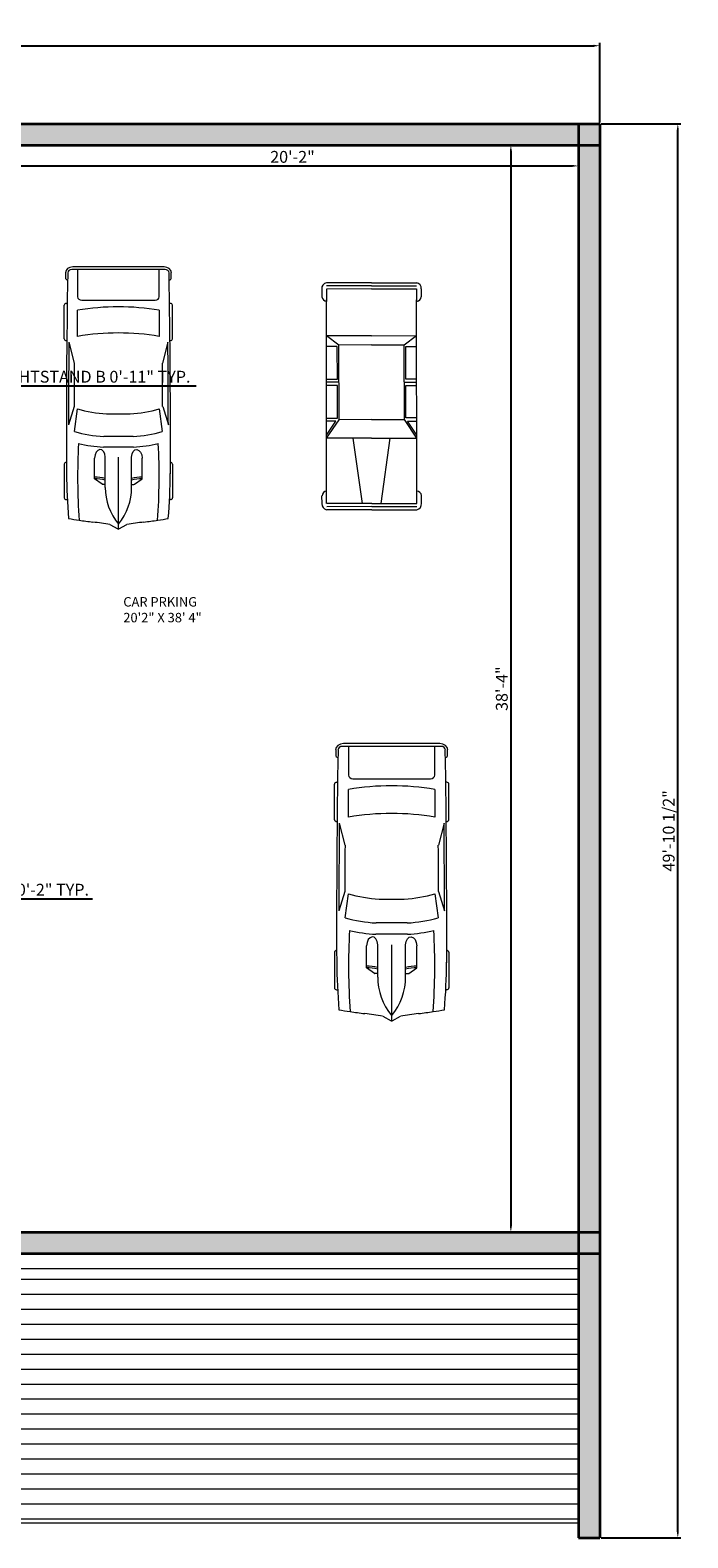
# Model space of a CAD drawing. Units: millimetres. Extents: x 2768 to 4359, y 795 to 1583.
# Tile 5 of 13: x 3226 to 3505, y 891 to 1529. Entities that reach past the tile are written whole.
import ezdxf

# ---------------------------------------------------------------- set-up
doc = ezdxf.new("R2010")
doc.units = ezdxf.units.MM
for name, color, linetype, lineweight in [('A-ANNO-DIMS', 90, 'Continuous', 18), ('A-AREA-IDEN', 190, 'Continuous', 18), ('A-DOOR-PATT', 251, 'Continuous', 13), ('A-WALL-PATT', 140, 'Continuous', 9), ('C-PKNG-VEHI', 50, 'Continuous', 13), ('iron shutter', 251, 'Continuous', 18), ('walls', 140, 'Continuous', 35)]:
    doc.layers.add(name, color=color, linetype=linetype, lineweight=lineweight)
doc.styles.get("Standard").update_dxf_attribs({"font": 'arial.ttf'})
doc.dimstyles.new('ISO-25', dxfattribs={"dimtxt": 5, "dimasz": 2.5, "dimexe": 1.25, "dimexo": 0.625, "dimtad": 1, "dimdec": 0, "dimlunit": 3, "dimtxsty": 'Standard', "dimcen": 2.5, "dimadec": 0, "dimazin": 0, "dimtfac": 1, "dimtdec": 0, "dimtmove": 0, "dimatfit": 3, "dimfxl": 1, "dimarcsym": 0})

# ---------------------------------------------------------------- blocks, each defined once
blk = doc.blocks.new('*U34')
for p, q in [((21.1, 37.4), (21.1, 36.8)), ((46.6, 38.9), (22.4, 38.9)), ((47.8, 37.4), (47.8, 37.4)), ((70, 31.5), (86.4, 29.4)), ((88, 31.9), (74.8, 35.9)), ((134.3, 35.6), (119.3, 31.8)), ((135.5, 37.1), (135.5, 37.4)), ((136.7, 38.9), (160.9, 38.9)), ((162.1, 37.4), (162.1, 36.8)), ((186.5, -33.5), (186.5, 33.5)), ((188.4, -32.8), (188.4, 32.8)), ((138.4, 29.4), (157.2, 29.4)), ((164.5, 26.4), (164.5, -26.4)), ((186.5, 29.4), (167, 29.4)), ((32.1, 9.5), (32.1, 11.2)), ((32.3, 11.6), (36.1, 17.2)), ((36.1, 17.2), (50.9, 17.2)), ((58.9, -10.8), (58.9, 10.8)), ((66.6, -10.5), (66.6, 10.5)), ((186.5, -10.5), (186.5, 10.5)), ((3.3, 6.1), (0.1, 0.4)), ((29.8, 9.5), (51.7, 9.5)), ((82.7, 8.5), (82.7, -8.5)), ((0, 0), (51.7, 0)), ((0.1, -0.4), (3.3, -6.1)), ((29.8, -9.5), (51.7, -9.5)), ((32.1, -9.5), (32.1, -11.2)), ((32.3, -11.6), (36.1, -17.2)), ((36.1, -17.2), (50.9, -17.2)), ((86.4, -29.4), (70, -31.5)), ((157.2, -29.4), (138.4, -29.4)), ((167, -29.4), (186.5, -29.4)), ((21.1, -37.4), (21.1, -36.8)), ((46.6, -38.9), (22.4, -38.9)), ((47.8, -37.4), (47.8, -37.4)), ((88, -31.9), (74.8, -35.9)), ((134.3, -35.6), (119.3, -31.8)), ((135.5, -37.1), (135.5, -37.4)), ((136.7, -38.9), (160.9, -38.9)), ((162.1, -37.4), (162.1, -36.8))]:
    blk.add_line(p, q)
for centre, major_axis, ratio, start_param, end_param in [((266, -27.5), (0, 313.3), 0.842304, 1.367076, 1.39176), ((41.2, -490.9), (0, 528.2), 0.842304, 0.00281, 0.075598), ((22.4, 37.4), (0, -1.48), 0.842304, 3.141593, 4.712389), ((64.5, -10555.6), (0, 10593), 0.842304, -0.013397, 0.002797), ((46.6, 37.4), (0, 1.48), 0.842304, -1.570796, 0), ((135.3, 5.4), (0, 81.8), 0.842304, 1.245306, 1.50788), ((64.5, -10555.6), (0, -10591.5), 0.842304, 3.133765, 3.140441), ((95.8, -3666.4), (0, -3698.2), 0.842304, 3.134049, 3.144098), ((136.7, 37.4), (0, -1.48), 0.842304, 3.141593, 4.712389), ((160.9, 37.4), (0, 1.48), 0.842304, -1.570796, 0), ((180.6, 35.8), (0, 2.22), 0.842304, -0.013017, 1.249894), ((64.5, -10556.4), (0, 10595.3), 0.842304, -0.013397, -0.013017), ((184, 32.8), (0, -5.25), 0.842304, 1.570796, 3.128196), ((184, 33.5), (0, -2.96), 0.842304, 1.570796, 3.128196), ((259.2, -27.5), (0, -305.3), 0.842304, 4.528606, 4.561838), ((37.5, -594), (0, -623.3), 0.842304, 3.096046, 3.200911), ((134.4, 5.4), (0, -89.8), 0.842304, 4.449482, 4.652344), ((149.6, 2.8), (0, -79.6), 0.842304, 4.372215, 4.640744), ((17.1, 0), (0, 147), 0.842304, 4.511394, 4.913384), ((35.9, 0), (0, 147), 0.842304, 4.511394, 4.913384), ((167, 26.4), (0, 2.96), 0.842304, 0, 1.570796), ((-204.5, 52.4), (0, -251), 0.842304, 1.385369, 1.434372), ((32.7, 11.2), (0, 0.74), 0.842304, 0.879714, 1.570796), ((13, 17), (0, 27.4), 0.842304, 4.435146, 4.718221), ((14.2, 17), (0, 27.4), 0.842304, 4.435146, 4.718221), ((50.8, 13.3), (6.34, -0.36), 0.603834, -1.395552, 1.581315), ((0.6, 0), (0, -0.74), 0.842304, 4.131459, 5.293319), ((29.8, -46.7), (0, 56.2), 0.842304, 0, 0.590319), ((-204.5, -52.4), (0, 251), 0.842304, -1.434372, -1.385369), ((29.8, 46.7), (0, 56.2), 0.842304, 2.551274, 3.141593), ((13, -17), (0, -27.4), 0.842304, 1.564964, 1.848039), ((14.2, -17), (0, -27.4), 0.842304, 1.564964, 1.848039), ((149.6, -2.8), (0, -79.6), 0.842304, -1.499151, -1.230623), ((259.2, 27.5), (0, 305.3), 0.842304, 1.721348, 1.754579), ((32.7, -11.2), (0, -0.74), 0.842304, 4.712389, 5.403472), ((134.4, -5.4), (0, -89.8), 0.842304, -1.510751, -1.307889), ((135.3, -5.4), (0, -81.8), 0.842304, -1.50788, -1.245306), ((266, 27.5), (0, 313.3), 0.842304, 1.749832, 1.774517), ((37.5, 594), (0, -623.3), 0.842304, -0.059319, 0.045547), ((167, -26.4), (0, -2.96), 0.842304, 4.712389, 6.283185), ((41.2, 490.9), (0, -528.2), 0.842304, -0.075598, -0.00281), ((22.4, -37.4), (0, 1.48), 0.842304, 1.570796, 3.141593), ((64.5, 10555.6), (0, 10593), 0.842304, 3.138796, 3.15499), ((46.6, -37.4), (0, -1.48), 0.842304, 0, 1.570796), ((64.5, 10555.6), (0, -10591.5), 0.842304, 0.001152, 0.007828), ((95.8, 3666.4), (0, -3698.2), 0.842304, -0.002505, 0.007544), ((136.7, -37.4), (0, -1.48), 0.842304, -1.570796, 0), ((160.9, -37.4), (0, 1.48), 0.842304, 3.141593, 4.712389), ((180.6, -35.8), (0, -2.22), 0.842304, -1.249894, 0.013017), ((64.5, 10556.4), (0, 10595.3), 0.842304, 3.15461, 3.15499), ((184, -32.8), (0, -5.25), 0.842304, 0.013397, 1.570796), ((184, -33.5), (0, 2.96), 0.842304, 3.15499, 4.712389)]:
    blk.add_ellipse(centre, major_axis=major_axis, ratio=ratio, start_param=start_param, end_param=end_param)
at = {"extrusion": (0, 0, -1)}
blk.add_ellipse((50.8, -13.3), major_axis=(6.34, 0.36), ratio=0.603834, start_param=-1.395552, end_param=1.581315, dxfattribs=at)
blk = doc.blocks.new('*U35')
for p, q in [((5.4, 42.3), (12.1, 42.3)), ((189.7, 42.3), (183, 42.3)), ((0.1, -0.4), (0.1, 38.3)), ((2.8, -0.4), (2.8, 38.3)), ((5.4, 38.3), (16.1, 38.3)), ((5.4, -0.4), (5.4, 38.2)), ((16.1, 38.3), (180.3, 38.3)), ((61.5, -0.4), (61.5, 38.3)), ((61.5, 38.3), (77.5, 27.6)), ((64.2, 38.3), (76.2, 30.3)), ((76.2, 30.3), (76.2, 38.3)), ((77.5, 27.6), (141.6, 27.6)), ((77.5, -0.4), (77.5, 27.6)), ((78.9, 38.3), (78.9, 29)), ((78.9, 29), (106.9, 29)), ((106.9, 29), (106.9, 38.3)), ((109.6, 27.6), (109.6, 38.3)), ((112.3, 38.3), (112.3, 29)), ((112.3, 29), (140.3, 29)), ((140.3, 29), (140.3, 38.3)), ((141.6, 27.6), (149.6, 38.3)), ((141.6, -0.4), (141.6, 27.6)), ((149.6, -0.4), (149.6, 38.3)), ((189.7, 38.3), (179, 38.3)), ((189.7, -0.4), (189.7, 38.2)), ((192.4, -0.4), (192.4, 38.3)), ((195, -0.4), (195, 38.3)), ((5.4, 7.6), (61.5, 15.6)), ((0.1, -0.4), (0.1, -39.2)), ((2.8, -0.4), (2.8, -39.1)), ((5.4, -0.4), (5.4, -39.1)), ((5.4, -8.4), (61.5, -16.4)), ((61.5, -0.4), (61.5, -39.1)), ((77.5, -0.4), (77.5, -28.5)), ((141.6, -0.4), (141.6, -28.5)), ((149.6, -0.4), (149.6, -39.1)), ((189.7, -0.4), (189.7, -39.1)), ((192.4, -0.4), (192.4, -39.1)), ((195, -0.4), (195, -39.2)), ((61.5, -39.1), (77.5, -28.5)), ((64.2, -39.1), (76.2, -31.1)), ((76.2, -31.1), (76.2, -39.1)), ((77.5, -28.5), (141.6, -28.5)), ((78.9, -39.1), (78.9, -29.8)), ((78.9, -29.8), (106.9, -29.8)), ((106.9, -29.8), (106.9, -39.1)), ((109.6, -28.5), (109.6, -39.1)), ((112.3, -29.8), (140.3, -29.8)), ((112.3, -39.1), (112.3, -29.8)), ((140.3, -29.8), (140.3, -39.1)), ((141.6, -28.5), (149.6, -39.1)), ((5.4, -39.1), (16.1, -39.1)), ((5.4, -43.1), (12.1, -43.1)), ((16.1, -39.1), (180.3, -39.1)), ((189.7, -39.1), (179, -39.1)), ((189.7, -43.1), (183, -43.1))]:
    blk.add_line(p, q)
for centre, radius, start, end in [((5.1, 37.3), 5.06, 85.6455, 168.0943), ((11.5, 37.6), 4.72, 8.1301, 81.87), ((183.7, 37.6), 4.72, 98.13, 171.8699), ((190.1, 37.3), 5.06, 11.9057, 94.3545), ((5.1, -38.1), 5.06, 191.9057, 274.3545), ((11.5, -38.5), 4.72, 278.13, 351.8699), ((183.7, -38.5), 4.72, 188.1301, 261.87), ((190.1, -38.1), 5.06, 265.6455, 348.0943)]:
    blk.add_arc(centre, radius, start, end)
blk = doc.blocks.new('*D36')
at = {"layer": 'A-ANNO-DIMS', "color": 0, "lineweight": -2, "transparency": 16777216}
for p, q in [((3216.41, 1480.21), (3216.41, 1470.35)), ((3458.41, 1480.21), (3458.41, 1470.35)), ((3218.91, 1471.6), (3455.91, 1471.6))]:
    blk.add_line(p, q, dxfattribs=at)
at = {"layer": 'A-ANNO-DIMS', "color": 0, "transparency": 16777216}
for points in [[(3218.91, 1472.02), (3218.91, 1471.19), (3216.41, 1471.6)], [(3455.91, 1472.02), (3455.91, 1471.19), (3458.41, 1471.6)]]:
    blk.add_solid(points, dxfattribs=at)
at = {"layer": 'Defpoints', "color": 0, "transparency": 16777216}
for p in [(3216.41, 1480.83), (3458.41, 1480.83), (3458.41, 1471.6)]:
    blk.add_point(p, dxfattribs=at)
at = {"layer": 'A-ANNO-DIMS', "color": 0, "transparency": 16777216, "insert": (3337.41, 1474.78), "char_height": 5, "attachment_point": 5}
blk.add_mtext('20\'-2"', dxfattribs=at)
blk = doc.blocks.new('*D37')
at = {"layer": 'A-ANNO-DIMS', "color": 0, "lineweight": -2, "transparency": 16777216}
for p, q in [((3428.05, 1480.41), (3431.06, 1480.41)), ((3429.81, 1477.91), (3429.81, 1022.91)), ((3428.05, 1020.41), (3431.06, 1020.41))]:
    blk.add_line(p, q, dxfattribs=at)
at = {"layer": 'A-ANNO-DIMS', "color": 0, "transparency": 16777216}
for points in [[(3429.39, 1477.91), (3430.23, 1477.91), (3429.81, 1480.41)], [(3429.39, 1022.91), (3430.23, 1022.91), (3429.81, 1020.41)]]:
    blk.add_solid(points, dxfattribs=at)
at = {"layer": 'Defpoints', "color": 0, "transparency": 16777216}
for p in [(3427.42, 1480.41), (3427.42, 1020.41), (3429.81, 1020.41)]:
    blk.add_point(p, dxfattribs=at)
at = {"layer": 'A-ANNO-DIMS', "color": 0, "transparency": 16777216, "insert": (3426.63, 1250.41), "char_height": 5, "attachment_point": 5, "rotation": 90}
blk.add_mtext('38\'-4"', dxfattribs=at)
blk = doc.blocks.new('*D119')
at = {"layer": 'A-ANNO-DIMS', "color": 0, "lineweight": -2, "transparency": 16777216}
for p, q in [((3193.99, 1379.55), (3193.99, 1377.29)), ((3196.49, 1378.54), (3202.37, 1378.54)), ((3204.87, 1379.55), (3204.87, 1377.29)), ((3204.87, 1378.54), (3296.68, 1378.54))]:
    blk.add_line(p, q, dxfattribs=at)
at = {"layer": 'A-ANNO-DIMS', "color": 0, "transparency": 16777216}
for points in [[(3196.49, 1378.96), (3196.49, 1378.13), (3193.99, 1378.54)], [(3202.37, 1378.96), (3202.37, 1378.13), (3204.87, 1378.54)]]:
    blk.add_solid(points, dxfattribs=at)
at = {"layer": 'Defpoints', "color": 0, "transparency": 16777216}
for p in [(3193.99, 1380.18), (3204.87, 1380.18), (3204.87, 1378.54)]:
    blk.add_point(p, dxfattribs=at)
at = {"layer": 'A-ANNO-DIMS', "color": 0, "transparency": 16777216, "insert": (3252.03, 1381.75), "char_height": 5, "attachment_point": 5}
blk.add_mtext('NIGHTSTAND B 0\'-11" TYP.', dxfattribs=at)
blk = doc.blocks.new('*D121')
at = {"layer": 'A-ANNO-DIMS', "color": 0, "lineweight": -2, "transparency": 16777216}
for p, q in [((3192.58, 1161.48), (3190.08, 1161.48)), ((3195.08, 1161.48), (3196.87, 1161.48)), ((3195.08, 1161.12), (3195.08, 1160.23)), ((3196.87, 1161.12), (3196.87, 1160.23)), ((3199.37, 1161.48), (3252.74, 1161.48))]:
    blk.add_line(p, q, dxfattribs=at)
at = {"layer": 'A-ANNO-DIMS', "color": 0, "transparency": 16777216}
for points in [[(3192.58, 1161.9), (3192.58, 1161.06), (3195.08, 1161.48)], [(3199.37, 1161.9), (3199.37, 1161.06), (3196.87, 1161.48)]]:
    blk.add_solid(points, dxfattribs=at)
at = {"layer": 'Defpoints', "color": 0, "transparency": 16777216}
for p in [(3195.08, 1161.75), (3196.87, 1161.75), (3196.87, 1161.48)]:
    blk.add_point(p, dxfattribs=at)
at = {"layer": 'A-ANNO-DIMS', "color": 0, "transparency": 16777216, "insert": (3227.3, 1164.69), "char_height": 5, "attachment_point": 5}
blk.add_mtext('RING 0\'-2" TYP.', dxfattribs=at)
blk = doc.blocks.new('*D125')
at = {"layer": 'A-ANNO-DIMS', "color": 0, "lineweight": -2, "transparency": 16777216}
for p, q in [((2811.41, 1490.03), (2811.41, 1523.71)), ((2813.91, 1522.46), (3464.91, 1522.46)), ((3467.41, 1490.03), (3467.41, 1523.71))]:
    blk.add_line(p, q, dxfattribs=at)
at = {"layer": 'A-ANNO-DIMS', "color": 0, "transparency": 16777216}
for points in [[(2813.91, 1522.87), (2813.91, 1522.04), (2811.41, 1522.46)], [(3464.91, 1522.87), (3464.91, 1522.04), (3467.41, 1522.46)]]:
    blk.add_solid(points, dxfattribs=at)
at = {"layer": 'Defpoints', "color": 0, "transparency": 16777216}
for p in [(3467.41, 1522.46), (2811.41, 1489.41), (3467.41, 1489.41)]:
    blk.add_point(p, dxfattribs=at)
at = {"layer": 'A-ANNO-DIMS', "color": 0, "transparency": 16777216, "insert": (3139.41, 1525.63), "char_height": 5, "attachment_point": 5}
blk.add_mtext('54\'-8"', dxfattribs=at)
blk = doc.blocks.new('*D126')
at = {"layer": 'A-ANNO-DIMS', "color": 0, "lineweight": -2, "transparency": 16777216}
for p, q in [((3468.03, 1489.41), (3501.71, 1489.41)), ((3500.46, 893.59), (3500.46, 1486.91)), ((3468.03, 891.09), (3501.71, 891.09))]:
    blk.add_line(p, q, dxfattribs=at)
at = {"layer": 'A-ANNO-DIMS', "color": 0, "transparency": 16777216}
for points in [[(3500.04, 1486.91), (3500.87, 1486.91), (3500.46, 1489.41)], [(3500.04, 893.59), (3500.87, 893.59), (3500.46, 891.09)]]:
    blk.add_solid(points, dxfattribs=at)
at = {"layer": 'Defpoints', "color": 0, "transparency": 16777216}
for p in [(3467.41, 1489.41), (3500.46, 1489.41), (3467.41, 891.09)]:
    blk.add_point(p, dxfattribs=at)
at = {"layer": 'A-ANNO-DIMS', "color": 0, "transparency": 16777216, "insert": (3497.25, 1190.25), "char_height": 5, "attachment_point": 5, "rotation": 90}
blk.add_mtext('49\'-10 1/2"', dxfattribs=at)

msp = doc.modelspace()

# ---------------------------------------------------------------- hatches: boundary and pattern name
at = {"layer": 'A-DOOR-PATT'}
h = msp.add_hatch(dxfattribs=at)
h.set_pattern_fill('ANSI31', color=256, scale=1.99444, angle=-45, style=0)
h.paths.add_polyline_path([(3216.41, 1005.07), (3458.41, 1005.07), (3458.41, 897.42), (3216.41, 897.42)])
at = {"layer": 'A-WALL-PATT'}
h = msp.add_hatch(color=256, dxfattribs=at)
h.dxf.hatch_style = 1
h.paths.add_polyline_path([(2820.41, 1480.41), (2811.41, 1480.41), (2811.41, 1360.41), (2820.41, 1360.41)])
h.paths.add_polyline_path([(2820.41, 1489.41), (2811.41, 1489.41), (2811.41, 1480.41), (2820.41, 1480.41)])
h.paths.add_polyline_path([(2845.83, 1489.41), (2820.41, 1489.41), (2820.41, 1480.41), (2845.83, 1480.41)])
h.paths.add_polyline_path([(2940.41, 1489.41), (2894.95, 1489.41), (2894.95, 1480.41), (2940.41, 1480.41)])
h.paths.add_polyline_path([(2949.41, 1489.41), (2940.41, 1489.41), (2940.41, 1480.41), (2949.41, 1480.41)])
h.paths.add_polyline_path([(2949.41, 1480.41), (2940.41, 1480.41), (2940.41, 1433.68), (2943.15, 1433.68), (2949.41, 1433.68)])
h.paths.add_polyline_path([(2964.2, 1489.41), (2949.41, 1489.41), (2949.41, 1480.41), (2964.2, 1480.41)])
h.paths.add_polyline_path([(3018.41, 1489.41), (3009.41, 1489.41), (3009.41, 1480.41), (3018.41, 1480.41)])
h.paths.add_polyline_path([(3009.41, 1489.41), (2990.92, 1489.41), (2990.92, 1480.41), (3009.41, 1480.41)])
h.paths.add_polyline_path([(3018.41, 1480.41), (3009.41, 1480.41), (3009.41, 1384.41), (3018.41, 1384.41)])
h.paths.add_polyline_path([(3009.41, 1384.41), (2949.41, 1384.41), (2949.41, 1375.41), (3009.41, 1375.41)])
h.paths.add_polyline_path([(3018.41, 1384.41), (3009.41, 1384.41), (3009.41, 1375.41), (3018.41, 1375.41)])
h.paths.add_polyline_path([(2949.41, 1384.41), (2940.41, 1384.41), (2940.41, 1375.41), (2949.41, 1375.41)])
h.paths.add_polyline_path([(2949.41, 1413.64, -0.075856), (2943.15, 1412.69), (2940.41, 1412.69), (2940.41, 1384.41), (2949.41, 1384.41)])
h.paths.add_polyline_path([(2949.41, 1375.41), (2940.41, 1375.41), (2940.41, 1360.41), (2949.41, 1360.41)])
h.paths.add_polyline_path([(2949.41, 1360.41), (2940.41, 1360.41), (2940.41, 1351.41), (2949.41, 1351.41)])
h.paths.add_polyline_path([(2940.41, 1360.41), (2929.82, 1360.41, -0.054277), (2930.46, 1354.53), (2930.46, 1351.41), (2940.41, 1351.41)])
h.paths.add_polyline_path([(2903.16, 1354.53), (2903.16, 1360.41), (2895.41, 1360.41), (2895.41, 1351.41), (2903.16, 1351.41)])
h.paths.add_polyline_path([(2886.41, 1360.41), (2820.41, 1360.41), (2820.41, 1351.41), (2886.41, 1351.41)])
h.paths.add_polyline_path([(2895.41, 1360.41), (2886.41, 1360.41), (2886.41, 1351.41), (2895.41, 1351.41)])
h.paths.add_polyline_path([(2820.41, 1360.41), (2811.41, 1360.41), (2811.41, 1351.41), (2820.41, 1351.41)])
h.paths.add_polyline_path([(2820.41, 1351.41), (2811.41, 1351.41), (2811.41, 1213.41), (2820.41, 1213.41)])
h.paths.add_polyline_path([(2886.41, 1213.41), (2820.41, 1213.41), (2820.41, 1204.41), (2886.41, 1204.41)])
h.paths.add_polyline_path([(2820.41, 1213.41), (2811.41, 1213.41), (2811.41, 1204.41), (2820.41, 1204.41)])
h.paths.add_polyline_path([(2895.41, 1302), (2886.41, 1302), (2886.41, 1264.47), (2895.41, 1264.47)])
h.paths.add_polyline_path([(2934.05, 1209.82), (2934.05, 1213.41), (2895.41, 1213.41), (2895.41, 1204.41), (2934.59, 1204.41, -0.049949)])
h.paths.add_polyline_path([(2895.41, 1213.41), (2886.41, 1213.41), (2886.41, 1204.41), (2895.41, 1204.41)])
h.paths.add_polyline_path([(3078.41, 1384.41), (3018.41, 1384.41), (3018.41, 1375.41), (3078.41, 1375.41)])
h.paths.add_polyline_path([(3087.41, 1433.68), (3084.62, 1433.68), (3078.41, 1433.68), (3078.41, 1384.41), (3087.41, 1384.41)])
h.paths.add_polyline_path([(3087.41, 1384.41), (3078.41, 1384.41), (3078.41, 1375.41), (3087.41, 1375.41)])
h.paths.add_polyline_path([(3087.41, 1375.41), (3078.41, 1375.41), (3078.41, 1360.41), (3087.41, 1360.41)])
h.paths.add_polyline_path([(3087.41, 1360.41), (3078.41, 1360.41), (3078.41, 1351.41), (3087.41, 1351.41)])
h.paths.add_polyline_path([(3093.5, 1360.41), (3087.41, 1360.41), (3087.41, 1351.41), (3093.5, 1351.41), (3093.5, 1353.18)])
h.paths.add_polyline_path([(3207.41, 1360.41), (3119.82, 1360.41, -0.067042), (3120.8, 1353.18), (3120.8, 1351.41), (3207.41, 1351.41)])
h.paths.add_polyline_path([(3216.41, 1480.41), (3207.41, 1480.41), (3207.41, 1360.41), (3216.41, 1360.41)])
h.paths.add_polyline_path([(3216.41, 1360.41), (3207.41, 1360.41), (3207.41, 1351.41), (3216.41, 1351.41)])
h.paths.add_polyline_path([(3216.41, 1489.41), (3207.41, 1489.41), (3207.41, 1480.41), (3216.41, 1480.41)])
h.paths.add_polyline_path([(3207.41, 1489.41), (3167.11, 1489.41), (3167.11, 1480.41), (3207.41, 1480.41)])
h.paths.add_polyline_path([(3118.27, 1489.41), (3087.41, 1489.41), (3087.41, 1480.41), (3118.27, 1480.41)])
h.paths.add_polyline_path([(3087.41, 1489.41), (3078.41, 1489.41), (3078.41, 1480.41), (3087.41, 1480.41)])
h.paths.add_polyline_path([(3087.41, 1480.41), (3078.41, 1480.41), (3078.41, 1453.72, -0.07525), (3084.62, 1454.66), (3087.41, 1454.66)])
h.paths.add_polyline_path([(3078.41, 1489.41), (3058.65, 1489.41), (3058.65, 1480.41), (3078.41, 1480.41)])
h.paths.add_polyline_path([(3031.86, 1489.41), (3018.41, 1489.41), (3018.41, 1480.41), (3031.86, 1480.41)])
h.paths.add_polyline_path([(3458.41, 1489.41), (3216.41, 1489.41), (3216.41, 1480.41), (3458.41, 1480.41)])
h.paths.add_polyline_path([(3467.41, 1489.41), (3458.41, 1489.41), (3458.41, 1480.41), (3467.41, 1480.41)])
h.paths.add_polyline_path([(3467.41, 1480.41), (3458.41, 1480.41), (3458.41, 1020.41), (3467.41, 1020.41)])
h.paths.add_polyline_path([(3458.41, 1020.41), (3216.41, 1020.41), (3216.41, 1011.41), (3458.41, 1011.41)])
h.paths.add_polyline_path([(3467.41, 1020.41), (3458.41, 1020.41), (3458.41, 1011.41), (3467.41, 1011.41)])
h.paths.add_polyline_path([(3216.41, 1080.41), (3207.41, 1080.41), (3207.41, 1020.41), (3216.41, 1020.41)])
h.paths.add_polyline_path([(3216.41, 1020.41), (3207.41, 1020.41), (3207.41, 1011.41), (3216.41, 1011.41)])
h.paths.add_polyline_path([(3207.41, 1020.41), (3151.59, 1020.41), (3151.59, 1011.41), (3207.41, 1011.41)])
h.paths.add_polyline_path([(3216.41, 1185.41), (3207.41, 1185.41), (3207.41, 1089.41), (3216.41, 1089.41)])
h.paths.add_polyline_path([(3216.41, 1089.41), (3207.41, 1089.41), (3207.41, 1080.41), (3216.41, 1080.41)])
h.paths.add_polyline_path([(3207.41, 1089.41), (3097.07, 1089.41), (3097.07, 1087.42), (3097.07, 1080.41), (3207.41, 1080.41)])
h.paths.add_polyline_path([(3216.41, 1194.41), (3207.41, 1194.41), (3207.41, 1185.41), (3216.41, 1185.41)])
h.paths.add_polyline_path([(3207.41, 1194.41), (3055.41, 1194.41), (3055.41, 1185.41), (3207.41, 1185.41)])
h.paths.add_polyline_path([(3055.41, 1194.41), (3046.41, 1194.41), (3046.41, 1185.41), (3055.41, 1185.41)])
h.paths.add_polyline_path([(3055.41, 1128.41), (3046.41, 1128.41), (3046.41, 1020.41), (3055.41, 1020.41)])
h.paths.add_polyline_path([(3055.41, 1020.41), (3046.41, 1020.41), (3046.41, 1011.41), (3055.41, 1011.41)])
h.paths.add_polyline_path([(3102.66, 1020.41), (3055.41, 1020.41), (3055.41, 1011.41), (3102.66, 1011.41)])
h.paths.add_polyline_path([(3055.41, 1137.41), (3046.41, 1137.41), (3046.41, 1128.41), (3055.41, 1128.41)])
h.paths.add_polyline_path([(3046.41, 1137.41), (2986.41, 1137.41), (2986.41, 1128.41), (3046.41, 1128.41)])
h.paths.add_polyline_path([(2986.41, 1204.41), (2977.41, 1204.41), (2977.41, 1137.41), (2986.41, 1137.41)])
h.paths.add_polyline_path([(2986.41, 1213.41), (2977.41, 1213.41), (2977.41, 1204.41), (2986.41, 1204.41)])
h.paths.add_polyline_path([(2977.41, 1213.41), (2961.35, 1213.41), (2961.35, 1209.82), (2961.35, 1204.41), (2977.41, 1204.41)])
h.paths.add_polyline_path([(2986.41, 1137.41), (2977.41, 1137.41), (2977.41, 1128.41), (2986.41, 1128.41)])
h.paths.add_polyline_path([(2986.41, 1128.41), (2977.41, 1128.41), (2977.41, 1073.04), (2980.14, 1073.04), (2986.41, 1073.04)])
h.paths.add_polyline_path([(2986.41, 1053, -0.075909), (2980.14, 1052.05), (2977.41, 1052.05), (2977.41, 1020.41), (2986.41, 1020.41)])
h.paths.add_polyline_path([(2986.41, 1020.41), (2977.41, 1020.41), (2977.41, 1011.41), (2986.41, 1011.41)])
h.paths.add_polyline_path([(2977.41, 1020.41), (2903.99, 1020.41), (2903.99, 1011.41), (2977.41, 1011.41)])
h.paths.add_polyline_path([(2820.41, 1111.04), (2811.41, 1111.04), (2811.41, 1020.41), (2820.41, 1020.41)])
h.paths.add_polyline_path([(2820.41, 1020.41), (2811.41, 1020.41), (2811.41, 1011.41), (2820.41, 1011.41)])
h.paths.add_polyline_path([(2855.32, 1020.41), (2820.41, 1020.41), (2820.41, 1011.41), (2855.32, 1011.41)])
h.paths.add_polyline_path([(2820.41, 1204.41), (2811.41, 1204.41), (2811.41, 1161.45), (2820.41, 1161.45)])
edge = h.paths.add_edge_path()
edge.add_arc((3211.84, 1295.2), 27.3, 86.96357, 99.35197)
edge.add_line((3207.41, 1322.13), (3207.41, 1351.41))
edge.add_line((3207.41, 1351.41), (3216.41, 1351.41))
edge.add_line((3216.41, 1351.41), (3216.41, 1322.29))
edge.add_line((3216.41, 1322.29), (3213.29, 1322.46))
h = msp.add_hatch(color=256, dxfattribs=at)
h.dxf.hatch_style = 1
h.paths.add_polyline_path([(3216.41, 1294.96), (3213.5, 1295.11), (3207.41, 1295.43), (3207.41, 1194.41), (3216.41, 1194.41)])
h.paths.add_polyline_path([(3216.41, 1011.41), (3207.41, 1011.41), (3207.41, 891.09), (3216.41, 891.09)])
h.paths.add_polyline_path([(3467.41, 1011.41), (3458.41, 1011.41), (3458.41, 891.09), (3467.41, 891.09)])

# ---------------------------------------------------------------- linework, layer by layer
at = {"layer": 'iron shutter'}
for p, q in [((3216.41, 1005.07), (3458.41, 1005.07)), ((3467.41, 916.42), (3467.41, 916.42)), ((3216.41, 897.42), (3458.41, 897.42))]:
    msp.add_line(p, q, dxfattribs=at)
at = {"layer": 'walls'}
for p, q in [((2811.41, 1489.41), (3467.41, 1489.41)), ((3458.41, 1489.41), (3458.41, 1011.41)), ((3467.41, 1489.41), (3467.41, 1011.41)), ((2811.41, 1480.41), (3467.41, 1480.41)), ((3055.41, 1020.41), (3467.41, 1020.41)), ((3055.41, 1011.41), (3467.41, 1011.41)), ((3458.41, 1011.41), (3458.41, 891.09)), ((3467.41, 1011.41), (3467.41, 891.09)), ((3458.41, 891.09), (3467.41, 891.09))]:
    msp.add_line(p, q, dxfattribs=at)

# ---------------------------------------------------------------- block references
at = {"layer": 'C-PKNG-VEHI'}
for name, p, xscale, yscale, zscale, rotation in [('*U34', (3263.75, 1317.96), 0.5886855226139459, 0.5886855226139459, 0.5886855226139459, 90), ('*U35', (3370.75, 1326.05), 0.4927787868258753, 0.4927787868258753, 0.4927787868258753, 90.06318951818653), ('*U34', (3379.38, 1109.82), 0.6229154369235925, 0.6229154369235925, 0.6229154369235925, 90)]:
    msp.add_blockref(name, p, dxfattribs=dict(at, xscale=xscale, yscale=yscale, zscale=zscale, rotation=rotation))

# ---------------------------------------------------------------- texts
at = {"layer": 'A-AREA-IDEN', "insert": (3265.82, 1289.14), "char_height": 4, "attachment_point": 1}
msp.add_mtext_dynamic_manual_height_columns('CAR PRKING \\P20\'2" X 38\' 4"', width=105.8375, gutter_width=12.5, heights=[0], dxfattribs=at)

# ---------------------------------------------------------------- dimensions: what is measured, and where the dimension line sits
at = {"layer": 'A-ANNO-DIMS'}
for base, p1, p2, override, picture, middle in [((3467.41, 1522.46), (2811.41, 1489.41), (3467.41, 1489.41), {"dimdec": 1, "dimlfac": 1, "dimrnd": 0, "dimzin": 1, "dimdsep": 46, "dimlunit": 4, "dimfrac": 2}, '*D125', (3139.41, 1525.63)), ((3458.41, 1471.6), (3216.41, 1480.83), (3458.41, 1480.83), {"dimclrd": 0, "dimclre": 0, "dimclrt": 0}, '*D36', (3337.41, 1474.78))]:
    dim = msp.add_linear_dim(base=base, p1=p1, p2=p2, dimstyle='ISO-25', override=override, dxfattribs=at)
    dim.commit()
    dim.dimension.update_dxf_attribs({"geometry": picture, "text_midpoint": middle})
for base, p1, p2, override, picture, middle in [((3500.46, 1489.41), (3467.41, 891.09), (3467.41, 1489.41), {"dimdec": 1, "dimlfac": 1, "dimrnd": 0, "dimzin": 1, "dimdsep": 46, "dimlunit": 4, "dimfrac": 2}, '*D126', (3497.25, 1190.25)), ((3429.81, 1020.41), (3427.42, 1480.41), (3427.42, 1020.41), {"dimclrd": 0, "dimclre": 0, "dimclrt": 0}, '*D37', (3426.63, 1250.41))]:
    dim = msp.add_linear_dim(base=base, p1=p1, p2=p2, angle=90, dimstyle='ISO-25', override=override, dxfattribs=at)
    dim.commit()
    dim.dimension.update_dxf_attribs({"geometry": picture, "text_midpoint": middle})
for base, p1, p2, text, picture, middle in [((3204.87, 1378.54), (3193.99, 1380.18), (3204.87, 1380.18), 'NIGHTSTAND B <> TYP.', '*D119', (3252.03, 1381.75)), ((3196.87, 1161.48), (3195.08, 1161.75), (3196.87, 1161.75), 'RING <> TYP.', '*D121', (3227.3, 1164.69))]:
    dim = msp.add_linear_dim(base=base, p1=p1, p2=p2, text=text, dimstyle='ISO-25', override={"dimdec": 1, "dimlfac": 1, "dimrnd": 0, "dimzin": 1, "dimdsep": 46, "dimlunit": 4, "dimfrac": 2}, dxfattribs=at)
    dim.commit()
    dim.dimension.update_dxf_attribs({"geometry": picture, "text_midpoint": middle})

doc.saveas('drawing.dxf')
